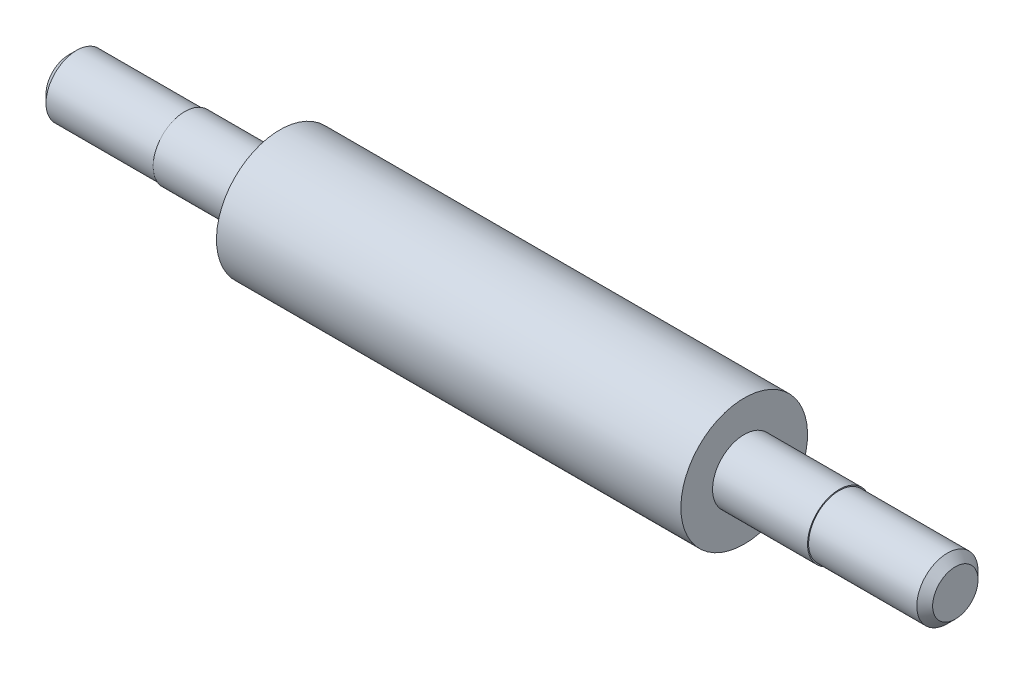
SolidWorks part; units mm, degrees
material "Plain Carbon Steel"
ref_plane "Front Plane" through (0, 0, 0) normal (0, 0, 1) x (1, 0, 0)
ref_plane "Top Plane" through (0, 0, 0) normal (0, 1, 0) x (1, 0, 0)
ref_plane "Right Plane" through (0, 0, 0) normal (1, 0, 0) x (0, 0, -1)
sketch "Shaft Profile Sketch" plane through (0, 0, 0) normal (0, 0, 1) x (1, 0, 0)
  line L0 (-420, 0) -> (1254.47, 0) construction
  line L1 (220, 60) -> (-220, 60)
  line L2 (220, 60) -> (220, 30)
  line L4 (-220, 60) -> (-220, 30)
  line L6 (-420, 0) -> (420, 0)
  line L7 (-220, 30) -> (-310, 30)
  line L10 (-310, 30) -> (-310, 29)
  line L13 (-310, 29) -> (-420, 29)
  line L16 (-420, 29) -> (-420, 0)
  line L19 (310, 30) -> (220, 30)
  line L20 (310, 30) -> (310, 29)
  line L25 (420, 29) -> (310, 29)
  line L26 (420, 29) -> (420, 0)
  point P0 (0, 0)
  point P6 (-220, 0)
  point P11 (-310, 0)
  point P16 (220, 0)
  point P21 (310, 0)
  dimension "D1" = 440
  dimension "D2" = 30
  dimension "D3" = 90
  dimension "D4" = 90
  dimension "D5" = 29
  dimension "D6" = 110
  dimension "D7" = 110
  dimension "D8" = 30
  dimension "D9" = 29
  dimension "D10" = 60
  dimension "D11" = 220
revolve "Stepped Shaft Body" add sketch "Shaft Profile Sketch" angle 360 about L0
chamfer "End Chamfer 7.5x45°" distance 7.5 angle 45 2 edges at (420, -29, 0) (-420, -29, 0)
